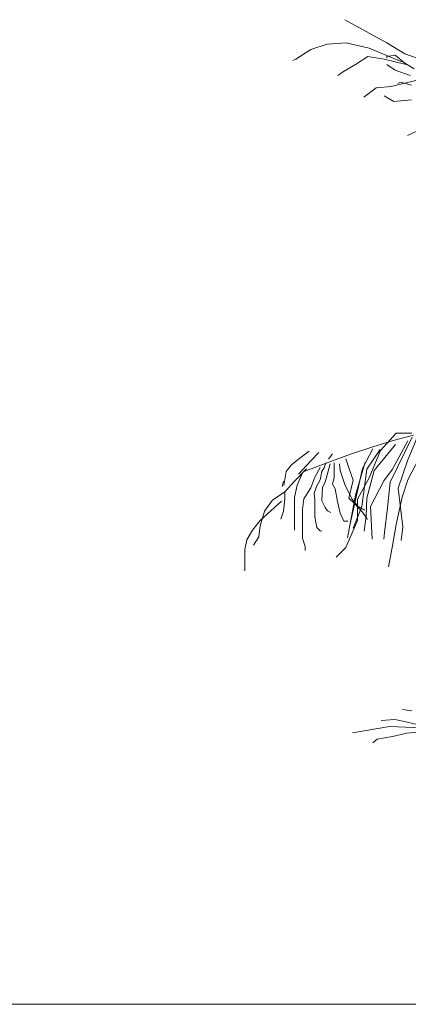
# Model space of a CAD drawing. Units: millimetres. Extents: x 595116 to 630915, y 909473 to 920225.
# Tile 95 of 134: x 629791.02 to 629798.32, y 919160.92 to 919179.41. Entities that reach past the tile are written whole.
import ezdxf

# ---------------------------------------------------------------- set-up
doc = ezdxf.new("R2010")
doc.units = ezdxf.units.MM
doc.layers.add('L-PLNT', color=85, linetype='Continuous', lineweight=13)

# ---------------------------------------------------------------- blocks, each defined once
blk = doc.blocks.new('A$C4FB75ABC')
for p, q in [((0.4999, 4.2779), (0.7111, 4.1621)), ((0.4114, 4.1553), (0.3296, 4.1281)), ((0.5068, 4.1621), (0.4114, 4.1553)), ((0.6226, 4.1349), (0.5068, 4.1621)), ((0.7111, 4.1621), (0.7997, 4.1076)), ((0.3296, 4.1281), (0.2547, 4.0804)), ((0.6158, 4.094), (0.5544, 4.0532)), ((0.6975, 4.0804), (0.6158, 4.094)), ((0.7861, 4.0668), (0.6226, 4.1349)), ((0.752, 4.1008), (0.7111, 4.094)), ((0.7111, 4.094), (0.7111, 4.0872)), ((0.7997, 4.06), (0.752, 4.1008)), ((0.7997, 4.1076), (0.8951, 4.0736)), ((0.2547, 4.0804), (0.241, 4.0736)), ((0.5544, 4.0532), (0.4931, 4.0191)), ((0.8065, 4.0532), (0.6975, 4.0804)), ((0.7111, 4.0532), (0.752, 4.0259)), ((0.8474, 4.0327), (0.7997, 4.06)), ((0.4931, 4.0191), (0.4659, 3.9987)), ((0.752, 4.0259), (0.827, 3.9987)), ((0.7316, 3.9442), (0.6566, 3.9374)), ((0.8746, 3.9783), (0.7316, 3.9442)), ((0.7793, 3.9647), (0.7656, 3.9578)), ((0.8338, 3.951), (0.7793, 3.9647)), ((0.6566, 3.9374), (0.5953, 3.8897)), ((0.7452, 3.8693), (0.6975, 3.8966)), ((0.8338, 3.8761), (0.7452, 3.8693)), ((0.8133, 3.6991), (0.8883, 3.7331)), ((0.7422, 2.1723), (0.6405, 2.1416)), ((0.7572, 2.2091), (0.6795, 2.1218)), ((0.837, 2.1896), (0.7276, 1.9635)), ((0.8151, 2.1714), (0.7385, 2.0291)), ((0.8429, 2.1986), (0.7422, 2.1723)), ((0.8348, 2.2091), (0.7572, 2.2091)), ((0.8699, 2.2079), (0.8151, 2.0766)), ((0.2683, 2.0784), (0.3228, 2.1193)), ((0.6405, 2.1416), (0.5342, 2.1057)), ((0.64, 2.1313), (0.5889, 2.0328)), ((0.6765, 2.1276), (0.6108, 2.0291)), ((0.6795, 2.1218), (0.6213, 1.986)), ((0.7531, 2.1531), (0.6473, 2.0218)), ((0.9125, 2.1606), (0.8154, 1.9763)), ((0.2342, 2.0512), (0.2683, 2.0784)), ((0.2683, 2.0035), (0.3296, 2.0716)), ((0.3296, 2.0716), (0.3705, 2.1125)), ((0.4182, 2.0784), (0.4386, 2.1057)), ((0.5342, 2.1057), (0.4195, 2.0639)), ((0.505, 2.0802), (0.5196, 2.0364)), ((0.8151, 2.0766), (0.7677, 1.9343)), ((0.207, 2.0172), (0.2342, 2.0512)), ((0.3092, 2.0308), (0.2479, 1.9695)), ((0.4195, 2.0639), (0.2927, 2.0154)), ((0.3773, 2.0376), (0.3501, 1.9899)), ((0.3966, 2.0361), (0.3855, 2.0168)), ((0.4049, 2.0609), (0.3966, 2.0361)), ((0.427, 2.0554), (0.4021, 1.9643)), ((0.4463, 2.0609), (0.4463, 1.9892)), ((0.4739, 2.0554), (0.4767, 2.0223)), ((0.4767, 2.0223), (0.5015, 1.9478)), ((0.5196, 2.0364), (0.5415, 1.9744)), ((0.5889, 2.0328), (0.5232, 1.741)), ((0.6018, 2.0636), (0.5533, 1.8986)), ((0.6108, 2.0291), (0.5853, 1.8431)), ((0.6473, 2.0218), (0.6108, 1.8833)), ((0.7385, 2.0291), (0.6947, 1.9708)), ((0.195, 1.9478), (0.207, 2.0172)), ((0.2887, 2.0103), (0.2615, 1.9491)), ((0.3501, 1.9899), (0.3296, 1.9354)), ((0.3773, 1.9754), (0.3607, 1.945)), ((0.3855, 2.0168), (0.3773, 1.9754)), ((0.4463, 1.9892), (0.438, 1.9533)), ((0.5415, 1.9744), (0.5196, 1.8833)), ((0.6213, 1.986), (0.563, 1.8792)), ((0.6947, 1.9708), (0.629, 1.8431)), ((0.8154, 1.9763), (0.7863, 1.8889)), ((0.1865, 1.9422), (0.1934, 1.9695)), ((0.2479, 1.9695), (0.2002, 1.915)), ((0.2615, 1.9491), (0.2479, 1.8878)), ((0.3296, 1.9354), (0.2956, 1.881)), ((0.3607, 1.945), (0.3469, 1.9091)), ((0.3883, 1.9395), (0.3855, 1.8705)), ((0.4021, 1.9643), (0.3883, 1.9395)), ((0.438, 1.9533), (0.4518, 1.9312)), ((0.4518, 1.9312), (0.4629, 1.8677)), ((0.5015, 1.9478), (0.5374, 1.8788)), ((0.7276, 1.9635), (0.713, 1.8358)), ((0.7677, 1.9343), (0.7896, 1.741)), ((0.1389, 1.8742), (0.098, 1.8197)), ((0.2002, 1.915), (0.1389, 1.8742)), ((0.2002, 1.881), (0.1934, 1.8197)), ((0.2002, 1.915), (0.2002, 1.881)), ((0.2479, 1.8878), (0.2479, 1.8061)), ((0.2956, 1.881), (0.2887, 1.8265)), ((0.3469, 1.9091), (0.3497, 1.876)), ((0.3497, 1.876), (0.3497, 1.8512)), ((0.5196, 1.8833), (0.5524, 1.8541)), ((0.5533, 1.8986), (0.5339, 1.7919)), ((0.5374, 1.8788), (0.5678, 1.8429)), ((0.563, 1.8792), (0.563, 1.7725)), ((0.6108, 1.8833), (0.6072, 1.7957)), ((0.7863, 1.8889), (0.7572, 1.7531)), ((0.1844, 1.8695), (0.0777, 1.7725)), ((0.2887, 1.8265), (0.2887, 1.7516)), ((0.3497, 1.8512), (0.3497, 1.7904)), ((0.3855, 1.8705), (0.4021, 1.8374)), ((0.4021, 1.8374), (0.4132, 1.8208)), ((0.4629, 1.8677), (0.4767, 1.8098)), ((0.5853, 1.8431), (0.5415, 1.7337)), ((0.5524, 1.8541), (0.5853, 1.8176)), ((0.5678, 1.8429), (0.5982, 1.8236)), ((0.629, 1.8431), (0.6363, 1.679)), ((0.713, 1.8358), (0.6984, 1.7118)), ((0.098, 1.8197), (0.0775, 1.7448)), ((0.1934, 1.8197), (0.1797, 1.7788)), ((0.2479, 1.8061), (0.2479, 1.7448)), ((0.3497, 1.7904), (0.3607, 1.738)), ((0.4132, 1.8208), (0.4297, 1.8125)), ((0.4767, 1.8098), (0.496, 1.7684)), ((0.5339, 1.7919), (0.5145, 1.6852)), ((0.5853, 1.8176), (0.6072, 1.7884)), ((0.6072, 1.7957), (0.5962, 1.7191)), ((0.6072, 1.7884), (0.6144, 1.7775)), ((0.0777, 1.7725), (0.0388, 1.724)), ((0.0775, 1.7448), (0.0707, 1.6903)), ((0.2479, 1.7448), (0.2479, 1.7243)), ((0.2887, 1.7516), (0.2887, 1.6835)), ((0.3607, 1.738), (0.3773, 1.7214)), ((0.496, 1.7684), (0.5153, 1.7684)), ((0.563, 1.7725), (0.5048, 1.6367)), ((0.7572, 1.7531), (0.7377, 1.6367)), ((0.7896, 1.741), (0.7823, 1.6717)), ((0.0097, 1.6755), (0, 1.627)), ((0.0388, 1.724), (0.0097, 1.6755)), ((0.0707, 1.6903), (0.0435, 1.6494)), ((0.2887, 1.6835), (0.3024, 1.6426)), ((0.3773, 1.7214), (0.3855, 1.7187)), ((0.6984, 1.7118), (0.6947, 1.679)), ((0, 1.627), (0, 1.5494)), ((0.3024, 1.6426), (0.3024, 1.6222)), ((0.5048, 1.6367), (0.4562, 1.5882)), ((0.7377, 1.6367), (0.7183, 1.5397)), ((0, 1.5494), (0, 1.5203)), ((0.8346, 0.8198), (0.7888, 0.827)), ((0.7236, 0.7411), (0.5379, 0.7092)), ((0.7503, 0.7767), (0.6814, 0.7711)), ((0.9219, 0.7334), (0.7236, 0.7411)), ((0.7912, 0.768), (0.7503, 0.7767)), ((0.8615, 0.7523), (0.7912, 0.768)), ((0.7393, 0.6917), (0.6621, 0.678)), ((0.8101, 0.7087), (0.7393, 0.6917)), ((0.879, 0.7143), (0.8101, 0.7087)), ((0.6621, 0.678), (0.6405, 0.6602))]:
    blk.add_line(p, q)

msp = doc.modelspace()

# ---------------------------------------------------------------- linework, layer by layer
at = {"layer": 'L-PLNT'}
msp.add_line((629511.274, 919160.917), (629824.951, 919160.917), dxfattribs=at)

# ---------------------------------------------------------------- block references
at = {"layer": 'L-PLNT', "xscale": 3.753413438031968, "yscale": 3.753413438031968, "zscale": 3.753413438031968}
msp.add_blockref('A$C4FB75ABC', (629795.248, 919163.35), dxfattribs=at)

doc.saveas('drawing.dxf')
